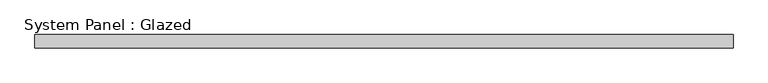
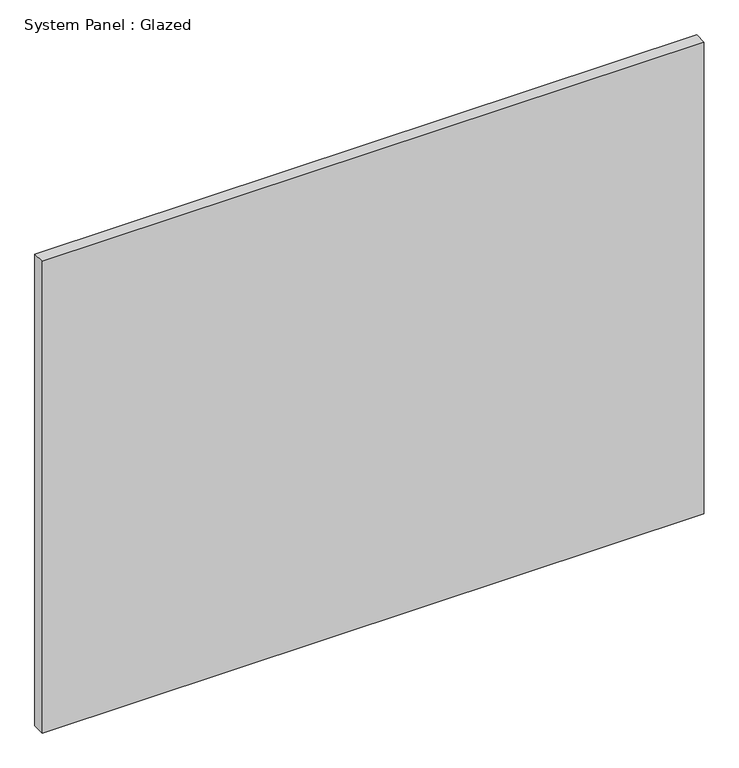
"""IFC4 building model written with IfcOpenShell, lengths in millimetres: plate geometry, System Panel : Glazed."""

from ifc_helpers import new_model, si_unit, origin, origin_with_axes, place, context, project, spatial, polyline, outline, extrude, source, transform, mapped, element, save


def system_panel_glazed_c2edcddf(model_context):
    return source(origin(), model_context, "Body", "SweptSolid", [
        extrude(outline(polyline([(661.32075, 19.05), (-661.32075, 19.05), (-661.32075, 44.45), (661.32075, 44.45), (661.32075, 19.05)])), origin_with_axes(), (0.0, 0.0, 1.0), 996.061),
    ])


if __name__ == "__main__":
    model = new_model("IFC4")
    model_context = context("Model", 3, world=origin())
    ifc_project = project(units=[si_unit("LENGTHUNIT", "METRE", prefix="MILLI")], contexts=[model_context])
    site = spatial("IfcSite", under=ifc_project)
    building = spatial("IfcBuilding", under=site)
    placement = place(None, origin())
    system_panel_glazed_shape = system_panel_glazed_c2edcddf(model_context)
    element("IfcPlate", 1, ObjectType="System Panel : Glazed", at=placement, inside=building, context=model_context, shape_type="MappedRepresentation", body=[
        mapped(system_panel_glazed_shape, transform((0.0, 0.0, 0.0), x_axis=(1.0, 0.0, 0.0), y_axis=(0.0, 1.0, 0.0), z_axis=(0.0, 0.0, 1.0))),
    ])
    save(model, "model.ifc")

# Revit data of these elements
# Type "System Panel : Glazed"
#   Construction Type Id = "GSP4R"
#   Analytic Construction = "1/8 in Pilkington single glazing"
#   Visual Light Transmittance = 0.9
#   Solar Heat Gain Coefficient = 0.86
#   Heat Transfer Coefficient (U) = 1.18115 BTU/(h·ft²·°F)
#   Define Thermal Properties by = 1
# Element 1 (IfcPlate, "System Panel : Glazed")
#   Materials on its faces: "Glass"
# Materials
#   "Glass": class "Glass", colour RGB 0 128 192, transparency 0.75, Description = "Soda Lime Glass", Cost = 0
